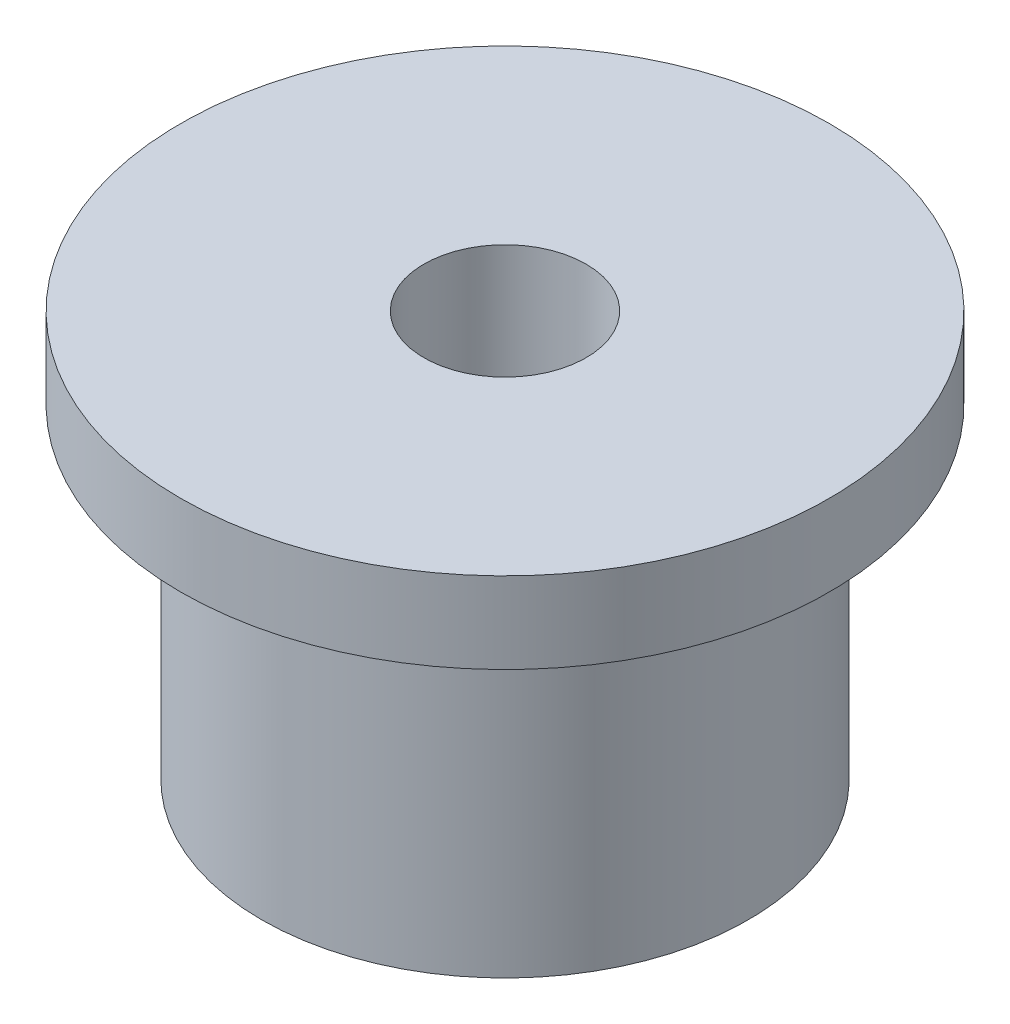
ISO-10303-21;
HEADER;
FILE_DESCRIPTION(('STEP AP214'),'2;1');
FILE_NAME('part.step','',(''),(''),'','','');
FILE_SCHEMA(('AUTOMOTIVE_DESIGN { 1 0 10303 214 1 1 1 1 }'));
ENDSEC;
DATA;
#1=APPLICATION_CONTEXT('core data for automotive mechanical design processes');
#2=APPLICATION_PROTOCOL_DEFINITION('international standard','automotive_design',2000,#1);
#3=PRODUCT_CONTEXT('',#1,'mechanical');
#4=PRODUCT('Part','Part','',(#3));
#5=PRODUCT_RELATED_PRODUCT_CATEGORY('part','',(#4));
#6=PRODUCT_DEFINITION_FORMATION('','',#4);
#7=PRODUCT_DEFINITION_CONTEXT('part definition',#1,'design');
#8=PRODUCT_DEFINITION('design','',#6,#7);
#9=PRODUCT_DEFINITION_SHAPE('','',#8);
#10=(LENGTH_UNIT() NAMED_UNIT(*) SI_UNIT(.MILLI.,.METRE.));
#11=(NAMED_UNIT(*) PLANE_ANGLE_UNIT() SI_UNIT($,.RADIAN.));
#12=(NAMED_UNIT(*) SI_UNIT($,.STERADIAN.) SOLID_ANGLE_UNIT());
#13=UNCERTAINTY_MEASURE_WITH_UNIT(LENGTH_MEASURE(1.E-05),#10,'distance_accuracy_value','');
#14=(GEOMETRIC_REPRESENTATION_CONTEXT(3) GLOBAL_UNCERTAINTY_ASSIGNED_CONTEXT((#13)) GLOBAL_UNIT_ASSIGNED_CONTEXT((#10,
#11,#12)) REPRESENTATION_CONTEXT('',''));
#15=CARTESIAN_POINT('',(0.,0.,0.));
#16=DIRECTION('',(0.,0.,1.));
#17=DIRECTION('',(1.,0.,0.));
#18=AXIS2_PLACEMENT_3D('',#15,#16,#17);
#19=CARTESIAN_POINT('',(0.,0.,-75.));
#20=DIRECTION('',(0.,-1.,0.));
#21=DIRECTION('',(0.,0.,-1.));
#22=AXIS2_PLACEMENT_3D('',#19,#20,#21);
#23=PLANE('',#22);
#24=CARTESIAN_POINT('',(0.,0.,0.));
#25=DIRECTION('',(0.,-1.,0.));
#26=DIRECTION('',(0.,0.,-1.));
#27=AXIS2_PLACEMENT_3D('',#24,#25,#26);
#28=CIRCLE('',#27,75.);
#29=CARTESIAN_POINT('',(0.,0.,-75.));
#30=VERTEX_POINT('',#29);
#31=EDGE_CURVE('E56',#30,#30,#28,.T.);
#32=ORIENTED_EDGE('',*,*,#31,.T.);
#33=EDGE_LOOP('',(#32));
#34=FACE_BOUND('',#33,.T.);
#35=CARTESIAN_POINT('',(0.,0.,0.));
#36=DIRECTION('',(0.,-1.,0.));
#37=DIRECTION('',(0.,0.,-1.));
#38=AXIS2_PLACEMENT_3D('',#35,#36,#37);
#39=CIRCLE('',#38,25.);
#40=CARTESIAN_POINT('',(0.,0.,-25.));
#41=VERTEX_POINT('',#40);
#42=EDGE_CURVE('E10',#41,#41,#39,.T.);
#43=ORIENTED_EDGE('',*,*,#42,.F.);
#44=EDGE_LOOP('',(#43));
#45=FACE_BOUND('',#44,.T.);
#46=ADVANCED_FACE('F40',(#34,#45),#23,.T.);
#47=CARTESIAN_POINT('',(0.,0.,0.));
#48=DIRECTION('',(0.,-1.,0.));
#49=DIRECTION('',(0.,0.,-1.));
#50=AXIS2_PLACEMENT_3D('',#47,#48,#49);
#51=CYLINDRICAL_SURFACE('',#50,25.);
#52=ORIENTED_EDGE('',*,*,#42,.T.);
#53=EDGE_LOOP('',(#52));
#54=FACE_BOUND('',#53,.T.);
#55=CARTESIAN_POINT('',(0.,125.,0.));
#56=DIRECTION('',(0.,-1.,0.));
#57=DIRECTION('',(0.,0.,-1.));
#58=AXIS2_PLACEMENT_3D('',#55,#56,#57);
#59=CIRCLE('',#58,25.);
#60=CARTESIAN_POINT('',(0.,125.,-25.));
#61=VERTEX_POINT('',#60);
#62=EDGE_CURVE('E43',#61,#61,#59,.T.);
#63=ORIENTED_EDGE('',*,*,#62,.F.);
#64=EDGE_LOOP('',(#63));
#65=FACE_BOUND('',#64,.T.);
#66=ADVANCED_FACE('F76',(#54,#65),#51,.F.);
#67=CARTESIAN_POINT('',(0.,125.,-25.));
#68=DIRECTION('',(0.,1.,0.));
#69=DIRECTION('',(0.,0.,1.));
#70=AXIS2_PLACEMENT_3D('',#67,#68,#69);
#71=PLANE('',#70);
#72=ORIENTED_EDGE('',*,*,#62,.T.);
#73=EDGE_LOOP('',(#72));
#74=FACE_BOUND('',#73,.T.);
#75=CARTESIAN_POINT('',(0.,125.,0.));
#76=DIRECTION('',(0.,-1.,0.));
#77=DIRECTION('',(0.,0.,-1.));
#78=AXIS2_PLACEMENT_3D('',#75,#76,#77);
#79=CIRCLE('',#78,100.);
#80=CARTESIAN_POINT('',(0.,125.,-100.));
#81=VERTEX_POINT('',#80);
#82=EDGE_CURVE('E50',#81,#81,#79,.T.);
#83=ORIENTED_EDGE('',*,*,#82,.F.);
#84=EDGE_LOOP('',(#83));
#85=FACE_BOUND('',#84,.T.);
#86=ADVANCED_FACE('F81',(#74,#85),#71,.T.);
#87=CARTESIAN_POINT('',(0.,0.,0.));
#88=DIRECTION('',(0.,-1.,0.));
#89=DIRECTION('',(0.,0.,-1.));
#90=AXIS2_PLACEMENT_3D('',#87,#88,#89);
#91=CYLINDRICAL_SURFACE('',#90,100.);
#92=ORIENTED_EDGE('',*,*,#82,.T.);
#93=EDGE_LOOP('',(#92));
#94=FACE_BOUND('',#93,.T.);
#95=CARTESIAN_POINT('',(0.,99.9999999999999,0.));
#96=DIRECTION('',(0.,-1.,0.));
#97=DIRECTION('',(0.,0.,-1.));
#98=AXIS2_PLACEMENT_3D('',#95,#96,#97);
#99=CIRCLE('',#98,100.);
#100=CARTESIAN_POINT('',(0.,99.9999999999999,-100.));
#101=VERTEX_POINT('',#100);
#102=EDGE_CURVE('E51',#101,#101,#99,.T.);
#103=ORIENTED_EDGE('',*,*,#102,.F.);
#104=EDGE_LOOP('',(#103));
#105=FACE_BOUND('',#104,.T.);
#106=ADVANCED_FACE('F71',(#94,#105),#91,.T.);
#107=CARTESIAN_POINT('',(0.,99.9999999999999,-100.));
#108=DIRECTION('',(0.,-1.,0.));
#109=DIRECTION('',(0.,0.,-1.));
#110=AXIS2_PLACEMENT_3D('',#107,#108,#109);
#111=PLANE('',#110);
#112=ORIENTED_EDGE('',*,*,#102,.T.);
#113=EDGE_LOOP('',(#112));
#114=FACE_BOUND('',#113,.T.);
#115=CARTESIAN_POINT('',(0.,99.9999999999999,0.));
#116=DIRECTION('',(0.,-1.,0.));
#117=DIRECTION('',(0.,0.,-1.));
#118=AXIS2_PLACEMENT_3D('',#115,#116,#117);
#119=CIRCLE('',#118,75.);
#120=CARTESIAN_POINT('',(0.,99.9999999999999,-75.));
#121=VERTEX_POINT('',#120);
#122=EDGE_CURVE('E57',#121,#121,#119,.T.);
#123=ORIENTED_EDGE('',*,*,#122,.F.);
#124=EDGE_LOOP('',(#123));
#125=FACE_BOUND('',#124,.T.);
#126=ADVANCED_FACE('F70',(#114,#125),#111,.T.);
#127=CARTESIAN_POINT('',(0.,0.,0.));
#128=DIRECTION('',(0.,-1.,0.));
#129=DIRECTION('',(0.,0.,-1.));
#130=AXIS2_PLACEMENT_3D('',#127,#128,#129);
#131=CYLINDRICAL_SURFACE('',#130,75.);
#132=ORIENTED_EDGE('',*,*,#122,.T.);
#133=EDGE_LOOP('',(#132));
#134=FACE_BOUND('',#133,.T.);
#135=ORIENTED_EDGE('',*,*,#31,.F.);
#136=EDGE_LOOP('',(#135));
#137=FACE_BOUND('',#136,.T.);
#138=ADVANCED_FACE('F62',(#134,#137),#131,.T.);
#139=CLOSED_SHELL('',(#46,#66,#86,#106,#126,#138));
#140=MANIFOLD_SOLID_BREP('B2',#139);
#141=ADVANCED_BREP_SHAPE_REPRESENTATION('',(#18,#140),#14);
#142=SHAPE_DEFINITION_REPRESENTATION(#9,#141);
ENDSEC;
END-ISO-10303-21;
